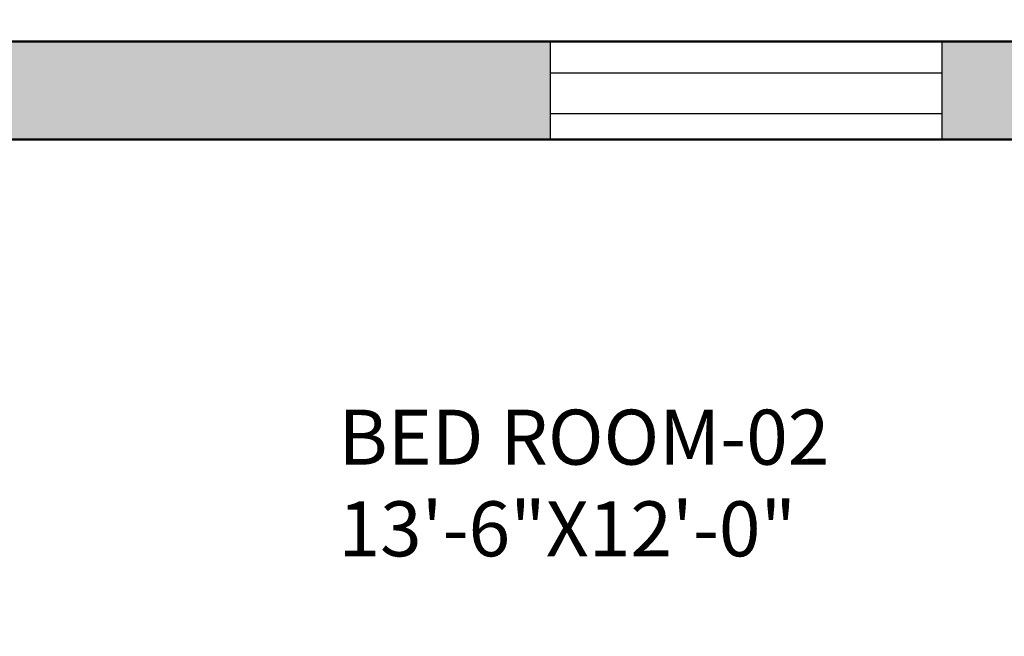
# Model space of a CAD drawing. Units: inches. Extents: x -7 to 1228, y -146 to 1091.
# Tile 79 of 88: x 654 to 744, y 946 to 1003. Entities that reach past the tile are written whole.
import ezdxf

# ---------------------------------------------------------------- set-up
doc = ezdxf.new("R2010")
doc.units = ezdxf.units.IN
for name, color, linetype, lineweight in [('A-AREA-IDEN', 7, 'Continuous', 18), ('A-GLAZ', 175, 'Continuous', 25), ('A-WALL', 7, 'Continuous', 50), ('A-WALL-PATT', 251, 'Continuous', 13)]:
    doc.layers.add(name, color=color, linetype=linetype, lineweight=lineweight)
doc.styles.get("Standard").update_dxf_attribs({"font": 'arial.ttf'})

# ---------------------------------------------------------------- blocks, each defined once
blk = doc.blocks.new('WIN-36')
for p, q in [((0, 36), (0, 0)), ((9, 36), (0, 36)), ((2.343, 36), (2.343, 0)), ((6.137, 0), (6.137, 36)), ((9, 0), (9, 36)), ((0, 0), (9, 0)), ((2.343, 0), (6.137, 0))]:
    blk.add_line(p, q)

msp = doc.modelspace()

# ---------------------------------------------------------------- hatches: boundary and pattern name
at = {"layer": 'A-WALL-PATT'}
h = msp.add_hatch(color=256, dxfattribs=at)
h.dxf.hatch_style = 1
h.paths.add_polyline_path([(69, 568), (60, 568), (60, 493), (63.289, 493), (69, 493)])
h.paths.add_polyline_path([(69, 662.405), (60, 662.405), (60, 586), (69, 586)], flags=17)
h.paths.add_polyline_path([(69, 723), (184, 723), (184, 734), (179, 734), (179, 728), (69, 728), (69, 741.623), (60, 741.623), (60, 698.405), (69, 698.405)], flags=17)
h.paths.add_polyline_path([(69, 782), (231, 782), (231, 728), (231, 723), (231, 586), (236, 586), (236, 787), (69, 787), (69, 800.126), (60, 800.126), (60, 765.623), (69, 765.623)])
h.paths.add_polyline_path([(184, 842), (189, 842), (189, 848), (173, 848), (173, 842), (179, 842), (179, 787), (184, 787)])
h.paths.add_polyline_path([(118.22, 69), (69, 69), (69, 60), (118.22, 60)])
h.paths.add_polyline_path([(227, 69), (154.22, 69), (154.22, 60), (227, 60)])
h.paths.add_polyline_path([(236, 60), (232.711, 60), (227, 60), (227, 36), (236, 36)])
h.paths.add_polyline_path([(389, 60), (380, 60), (380, 36), (389, 36)])
h.paths.add_polyline_path([(384, 181), (380, 181), (380, 115), (380, 78), (384, 78)])
h.paths.add_polyline_path([(380, 115), (334.547, 115), (334.547, 109), (380, 109)])
h.paths.add_polyline_path([(274.547, 115), (236, 115), (236, 201), (232.711, 201), (231, 201), (231, 78), (236, 78), (236, 109), (274.547, 109)])
h.paths.add_polyline_path([(69, 123), (60, 123), (60, 78), (69, 78)])
h.paths.add_polyline_path([(69, 201), (60, 201), (60, 159), (69, 159)])
h.paths.add_polyline_path([(143, 219), (69, 219), (69, 213), (143, 213)], flags=17)
h.paths.add_polyline_path([(189, 219), (184, 219), (184, 274), (231, 274), (231, 219), (236, 219), (236, 279), (184, 279), (184, 297), (179, 297), (179, 279), (69, 279), (69, 290.912), (60, 290.912), (60, 262.179), (69, 262.179), (69, 274), (179, 274), (179, 219), (173, 219), (173, 213), (189, 213)])
h.paths.add_polyline_path([(69, 238.179), (60, 238.179), (60, 219), (69, 219)], flags=17)
h.paths.add_polyline_path([(69, 333), (60, 333), (60, 314.912), (69, 314.912), (69, 316.965)])
h.paths.add_polyline_path([(190, 338), (184, 338), (69, 338), (69, 333), (179, 333), (179, 327), (184, 327), (184, 333.021), (190, 333.046)])
h.paths.add_polyline_path([(69, 386.806), (60, 386.806), (60, 351), (69, 351)])
h.paths.add_polyline_path([(69, 475), (60, 475), (60, 422.806), (69, 422.806)])
h.paths.add_polyline_path([(236, 475), (231, 475), (231, 351.238), (236, 351.238)])
h.paths.add_polyline_path([(384, 475), (380, 475), (380, 362), (384, 362)])
h.paths.add_polyline_path([(547, 307), (439, 307), (439, 356), (445, 356), (445, 362), (433, 362), (433, 307), (380, 307), (380, 244), (380, 241), (384, 241), (384, 301), (433, 301), (433, 277), (439, 277), (439, 301), (547, 301)])
h.paths.add_polyline_path([(547, 241), (439, 241), (439, 247), (433, 247), (433, 235), (547, 235)])
h.paths.add_polyline_path([(450, 69), (440.286, 69), (424.889, 69), (389, 69), (389, 60), (450, 60)])
h.paths.add_polyline_path([(547, 69), (486, 69), (486, 60), (547, 60)])
h.paths.add_polyline_path([(556, 148.268), (547, 148.268), (547, 78), (556, 78)])
h.paths.add_polyline_path([(556, 223), (547, 223), (547, 195), (547, 184.268), (556, 184.268)])
h.paths.add_polyline_path([(556, 311.192), (547, 311.192), (547, 273.075), (556, 273.075)])
h.paths.add_polyline_path([(556, 344), (552.711, 344), (547, 344), (547, 335.192), (556, 335.192)])
h.paths.add_polyline_path([(556, 249.075), (547, 249.075), (547, 241), (556, 241)])
h.paths.add_polyline_path([(547, 362), (475, 362), (475, 356), (547, 356)], flags=0)
h.paths.add_polyline_path([(556, 399.621), (547, 399.621), (547, 362), (556, 362)])
h.paths.add_polyline_path([(556, 475), (547, 475), (547, 435.621), (556, 435.621)])
h.paths.add_polyline_path([(547, 493), (389, 493), (389, 487), (547, 487)])
h.paths.add_polyline_path([(380, 493), (278, 493), (278, 487), (380, 487)])
h.paths.add_polyline_path([(227, 493), (69, 493), (69, 487), (227, 487)])
h.paths.add_polyline_path([(643, 122.445), (634, 122.445), (634, 78), (643, 78)])
h.paths.add_polyline_path([(702.5, 69), (692.786, 69), (677.389, 69), (643, 69), (643, 60), (702.5, 60)])
h.paths.add_polyline_path([(798, 69), (738.5, 69), (738.5, 60), (798, 60)])
h.paths.add_polyline_path([(807, 60), (803.711, 60), (798, 60), (798, 36), (807, 36)])
h.paths.add_polyline_path([(807, 109), (846.751, 109), (846.751, 115), (807, 115), (807, 159), (802, 159), (802, 78), (807, 78)])
h.paths.add_polyline_path([(807, 201), (802, 201), (802, 195), (807, 195)])
h.paths.add_polyline_path([(643, 201), (634, 201), (634, 158.445), (643, 158.445)])
h.paths.add_polyline_path([(756, 225), (751, 225), (751, 219), (643, 219), (643, 213), (756, 213)])
h.paths.add_polyline_path([(643, 240.848), (634, 240.848), (634, 219), (643, 219)])
h.paths.add_polyline_path([(643, 274), (643, 288.629), (634, 288.629), (634, 264.848), (643, 264.848)])
h.paths.add_polyline_path([(802, 279), (756, 279), (756, 297), (751, 297), (751, 279), (643, 279), (643, 274), (751, 274), (751, 255), (756, 255), (756, 274), (802, 274)])
h.paths.add_polyline_path([(807, 333), (803.711, 333), (802, 333), (802, 279), (802, 274), (802, 219), (807, 219)])
h.paths.add_polyline_path([(956, 182), (951, 182), (951, 115), (906.751, 115), (906.751, 109), (951, 109), (951, 78), (956, 78)])
h.paths.add_polyline_path([(960, 60), (951, 60), (951, 36), (960, 36)])
h.paths.add_polyline_path([(1021, 69), (1005.781, 69), (960, 69), (960, 60), (1021, 60)])
h.paths.add_polyline_path([(956, 224), (951, 224), (951, 218), (956, 218)])
h.paths.add_polyline_path([(956, 302), (1004, 302), (1004, 278), (1010, 278), (1010, 302), (1118, 302), (1118, 290.809), (1127, 290.809), (1127, 326.968), (1118, 326.968), (1118, 320.966), (1118, 307), (1010, 307), (1010, 356), (1016, 356), (1016, 362), (1004, 362), (1004, 307), (951, 307), (951, 244), (951, 242), (954.289, 242), (956, 242)])
h.paths.add_polyline_path([(643, 333), (634, 333), (634, 312.629), (643, 312.629), (643, 316.965)])
h.paths.add_polyline_path([(756, 338), (643, 338), (643, 333), (751, 333), (751, 327), (756, 327)])
h.paths.add_polyline_path([(643, 388), (634, 388), (634, 351), (643, 351)])
h.paths.add_polyline_path([(807, 357), (802, 357), (802, 351), (807, 351)])
h.paths.add_polyline_path([(807, 475), (802, 475), (802, 393), (807, 393)])
h.paths.add_polyline_path([(643, 475), (634, 475), (634, 424), (643, 424)])
h.paths.add_polyline_path([(798, 493), (643, 493), (643, 487), (798, 487)])
h.paths.add_polyline_path([(634, 493), (556, 493), (556, 487), (634, 487)])
h.paths.add_polyline_path([(813, 493), (807, 493), (807, 487), (813, 487)])
h.paths.add_polyline_path([(951, 493), (849, 493), (849, 487), (951, 487)])
h.paths.add_polyline_path([(956, 484), (951, 484), (951, 374), (956, 374)])
h.paths.add_polyline_path([(1109, 493), (969, 493), (969, 487), (1109, 487)])
h.paths.add_polyline_path([(1127, 484), (1118, 484), (1118, 450.641), (1127, 450.641)])
h.paths.add_polyline_path([(1127, 414.641), (1118, 414.641), (1118, 365), (1127, 365)])
h.paths.add_polyline_path([(1109, 362), (1046, 362), (1046, 356), (1109, 356)], flags=17)
h.paths.add_polyline_path([(1127, 356), (1123.454, 356), (1118, 356), (1118, 350.968), (1127, 350.968)], flags=0)
h.paths.add_polyline_path([(1127, 266.809), (1118, 266.809), (1118, 262.361), (1118, 242), (1127, 242)], flags=17)
h.paths.add_polyline_path([(1118, 242), (1010, 242), (1010, 248), (1004, 248), (1004, 237), (1118, 237)])
h.paths.add_polyline_path([(1127, 224), (1118, 224), (1118, 170), (1127, 170)])
h.paths.add_polyline_path([(1127, 134), (1118, 134), (1118, 78), (1127, 78)])
h.paths.add_polyline_path([(1118, 69), (1057, 69), (1057, 60), (1118, 60)])
h.paths.add_polyline_path([(227, 571.546), (227, 574), (69, 574), (69, 568), (227, 568)])
h.paths.add_polyline_path([(380, 571.546), (380, 574), (278, 574), (278, 568), (380, 568)])
h.paths.add_polyline_path([(242, 574), (236, 574), (236, 568), (242, 568)])
h.paths.add_polyline_path([(547, 571.546), (547, 574), (389, 574), (389, 568), (547, 568)])
h.paths.add_polyline_path([(384, 733), (380, 733), (380, 586), (384, 586)])
h.paths.add_polyline_path([(556, 646), (634, 646), (634, 655), (547, 655), (547, 586), (556, 586)])
h.paths.add_polyline_path([(634, 574), (556, 574), (556, 568), (634, 568)])
h.paths.add_polyline_path([(643, 655), (634, 655), (634, 586), (643, 586)])
h.paths.add_polyline_path([(798, 574), (643, 574), (643, 568), (798, 568)])
h.paths.add_polyline_path([(643, 663.854), (634, 663.854), (634, 655), (643, 655)])
h.paths.add_polyline_path([(556, 676.967), (547, 676.967), (547, 655), (556, 655)])
h.paths.add_polyline_path([(556, 733), (547, 733), (547, 712.967), (556, 712.967)])
h.paths.add_polyline_path([(643, 710), (634, 710), (634, 699.854), (643, 699.854)])
h.paths.add_polyline_path([(807, 668), (802, 668), (802, 586), (807, 586)])
h.paths.add_polyline_path([(951, 574), (849, 574), (849, 568), (951, 568)])
h.paths.add_polyline_path([(956, 691), (951, 691), (951, 577), (956, 577)])
h.paths.add_polyline_path([(1109, 574), (969, 574), (969, 568), (1109, 568)])
h.paths.add_polyline_path([(1127, 643.403), (1118, 643.403), (1118, 577), (1127, 577)])
h.paths.add_polyline_path([(1127, 568), (1123.454, 568), (1118, 568), (1118, 493), (1127, 493)])
h.paths.add_polyline_path([(1127, 733), (1118, 733), (1118, 679.403), (1127, 679.403)])
h.paths.add_polyline_path([(1127, 777.348), (1118, 777.348), (1118, 770.035), (1118, 751), (1127, 751)], flags=17)
h.paths.add_polyline_path([(1118, 751), (1010, 751), (1010, 757), (1004, 757), (1004, 745), (1118, 745)])
h.paths.add_polyline_path([(956, 811), (1004, 811), (1004, 787), (1010, 787), (1010, 811), (1017.874, 811), (1017.874, 811.627, -0.414214), (1018.247, 812), (1031.978, 812, -0.414214), (1032.351, 811.627), (1032.351, 811), (1118, 811), (1118, 801.348), (1127, 801.348), (1127, 834.685), (1118, 834.685), (1118, 830.238), (1118, 817), (1010, 817), (1010, 866), (1016, 866), (1016, 872), (1004, 872), (1004, 817), (956, 817), (956, 866), (951, 866), (951, 751), (954.289, 751), (956, 751)])
h.paths.add_polyline_path([(1118, 872), (1046, 872), (1046, 866), (1118, 866)], flags=17)
h.paths.add_polyline_path([(1127, 924.711), (1118, 924.711), (1118, 884), (1127, 884)])
h.paths.add_polyline_path([(1127, 866), (1123.711, 866), (1118, 866), (1118, 858.685), (1127, 858.685)], flags=17)
h.paths.add_polyline_path([(956, 983), (951, 983), (951, 952), (807, 952), (807, 983), (802, 983), (802, 902), (807, 902), (807, 946), (951, 946), (951, 884), (956, 884)])
h.paths.add_polyline_path([(807, 842), (802, 842), (802, 787), (756, 787), (756, 806), (751, 806), (751, 787), (643, 787), (643, 782), (751, 782), (751, 764), (756, 764), (756, 782), (802, 782), (802, 728), (807, 728)])
h.paths.add_polyline_path([(756, 848), (643, 848), (643, 842), (751, 842), (751, 836), (756, 836)])
h.paths.add_polyline_path([(756, 734), (751, 734), (751, 728), (643, 728), (643, 723), (756, 723)])
h.paths.add_polyline_path([(643, 749.791), (634, 749.791), (634, 728), (637.289, 728), (643, 728)])
h.paths.add_polyline_path([(643, 805.405), (634, 805.405), (634, 773.791), (643, 773.791)])
h.paths.add_polyline_path([(643, 896.663), (634, 896.663), (634, 860), (637.289, 860), (643, 860)])
h.paths.add_polyline_path([(643, 842), (634, 842), (634, 829.405), (643, 829.405)])
h.paths.add_polyline_path([(643, 983), (634, 983), (634, 932.663), (643, 932.663)])
h.paths.add_polyline_path([(1127, 983), (1118, 983), (1118, 960.711), (1127, 960.711)])
h.paths.add_polyline_path([(1118, 1001), (1077.525, 1001), (1077.525, 992), (1118, 992)])
h.paths.add_polyline_path([(1041.525, 1001), (960, 1001), (960, 992), (1041.525, 992)])
h.paths.add_polyline_path([(960, 1025), (951, 1025), (951, 1001), (954.289, 1001), (960, 1001)])
h.paths.add_polyline_path([(807, 1025), (798, 1025), (798, 1001), (807, 1001)])
h.paths.add_polyline_path([(798, 1001), (738.5, 1001), (738.5, 992), (798, 992)])
h.paths.add_polyline_path([(702.5, 1001), (643, 1001), (643, 992), (702.5, 992)])
h.paths.add_polyline_path([(547, 1001), (499.113, 1001), (499.113, 992), (547, 992)])
h.paths.add_polyline_path([(463.113, 1001), (389, 1001), (389, 992), (463.113, 992)])
h.paths.add_polyline_path([(389, 1025), (380, 1025), (380, 1022), (380, 1001), (383.289, 1001), (389, 1001)])
h.paths.add_polyline_path([(236, 1025), (227, 1025), (227, 1001), (236, 1001)])
h.paths.add_polyline_path([(236, 983), (231, 983), (231, 860), (236, 860)])
h.paths.add_polyline_path([(274.547, 952), (236, 952), (236, 946), (274.547, 946)])
h.paths.add_polyline_path([(380, 952), (334.547, 952), (334.547, 946), (380, 946)])
h.paths.add_polyline_path([(384, 983), (380, 983), (380, 884), (383.289, 884), (384, 884)])
h.paths.add_polyline_path([(227, 1001), (155.012, 1001), (155.012, 992), (162.875, 992), (227, 992)])
h.paths.add_polyline_path([(119.012, 1001), (69, 1001), (69, 992), (119.012, 992)])
h.paths.add_polyline_path([(69, 983), (60, 983), (60, 922.987), (69, 922.987)])
h.paths.add_polyline_path([(69, 886.987), (60, 886.987), (60, 860), (63.289, 860), (69, 860)])
h.paths.add_polyline_path([(143, 848), (69, 848), (69, 842), (143, 842)])

# ---------------------------------------------------------------- linework, layer by layer
at = {"layer": 'A-WALL'}
for p, q in [((807, 1001), (634, 1001)), ((807, 992), (634, 992))]:
    msp.add_line(p, q, dxfattribs=at)

# ---------------------------------------------------------------- block references
at = {"layer": 'A-GLAZ', "extrusion": (0, 0, -1), "zscale": -1, "rotation": 90.00000000000003}
msp.add_blockref('WIN-36', (-702.5, 992), dxfattribs=at)

# ---------------------------------------------------------------- texts
at = {"layer": 'A-AREA-IDEN', "insert": (682.994, 967.149), "char_height": 5.05676, "attachment_point": 1}
msp.add_mtext_dynamic_manual_height_columns('BED ROOM-02\\P13\'-6"X12\'-0"', width=137.28212, gutter_width=25.284, heights=[0], dxfattribs=at)

doc.saveas('drawing.dxf')
